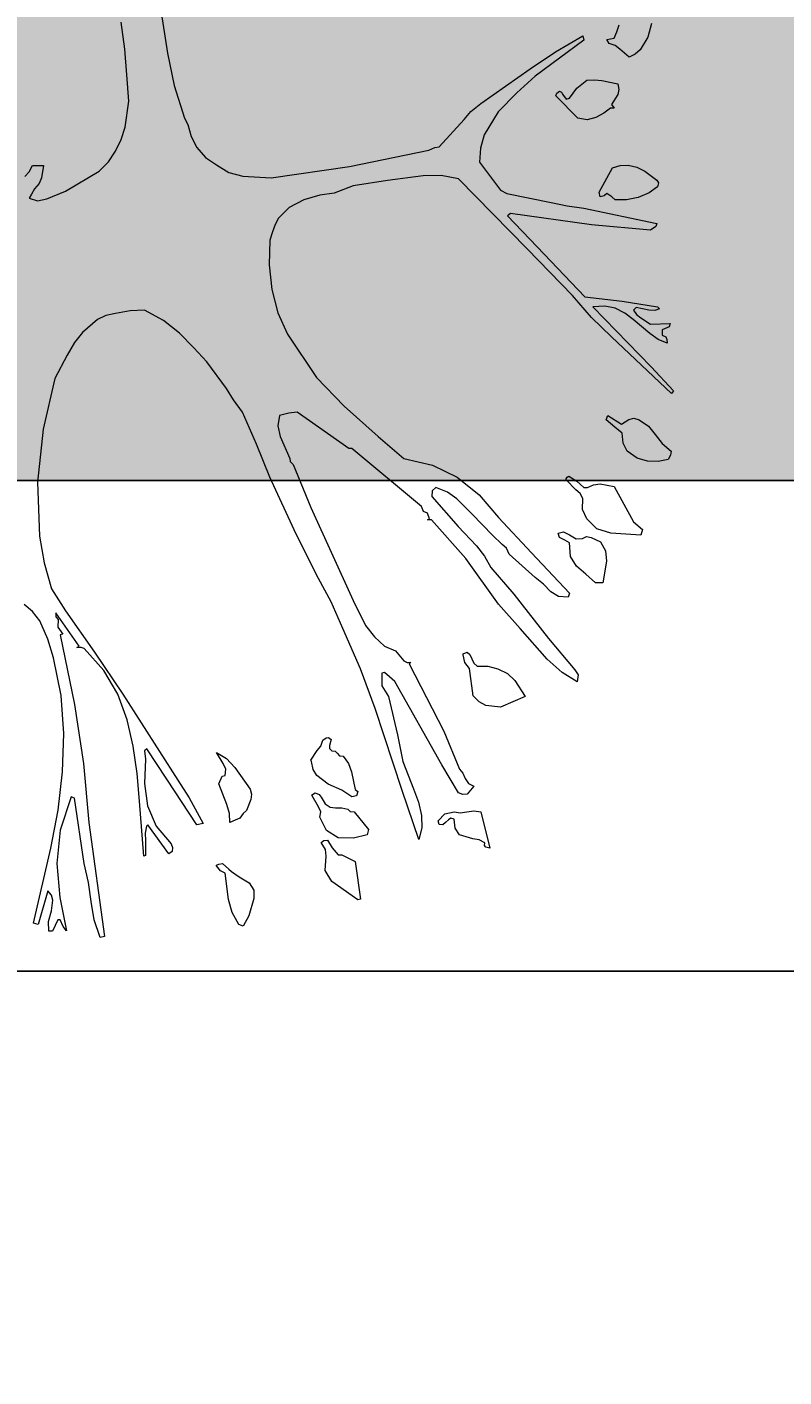
# Model space of a CAD drawing. Units: inches. Extents: x 84 to 1044, y -280 to 906.
# Tile 28 of 105: x 775 to 789, y -129 to -105. Entities that reach past the tile are written whole.
import ezdxf

# ---------------------------------------------------------------- set-up
doc = ezdxf.new("R2010")
doc.units = ezdxf.units.IN
for name, color, linetype, lineweight in [('A-ANNO-DIMS', 2, 'Continuous', 18), ('C-PROP', 7, 'Continuous', 25), ('L-PLNT', 114, 'Continuous', 15)]:
    doc.layers.add(name, color=color, linetype=linetype, lineweight=lineweight)
doc.layers.add('L-PLNT-PATT', color=9, linetype='Continuous', lineweight=9, true_color=0xafd9aa)
doc.styles.get("Standard").update_dxf_attribs({"font": 'arial.ttf'})
doc.dimstyles.get("Standard").update_dxf_attribs({"dimtxt": 0.18, "dimasz": 0.18, "dimexe": 0.18, "dimexo": 0.0625, "dimgap": 0.09, "dimtad": 0, "dimtih": 1, "dimtoh": 1, "dimdec": 4, "dimzin": 0, "dimdsep": 46, "dimtxsty": 'Standard', "dimcen": 0.09, "dimadec": 0, "dimazin": 0, "dimtfac": 1, "dimtdec": 4, "dimtofl": 0, "dimtmove": 0, "dimatfit": 3, "dimfxl": 1, "dimtolj": 1, "dimtzin": 0, "dimarcsym": 0})

# ---------------------------------------------------------------- blocks, each defined once
blk = doc.blocks.new('A$C37E508DF')
for p, q in [((0.7911, 1.1436), (0.8027, 1.0677)), ((0.7512, 1.0728), (0.7469, 1.1054)), ((1.3421, 1.0861), (1.3455, 1.0934)), ((1.3455, 1.0934), (1.3485, 1.102)), ((1.3875, 1.1037), (1.3828, 1.087)), ((1.3057, 1.0835), (1.2469, 1.0402)), ((1.2713, 1.0694), (1.3044, 1.0887)), ((1.3044, 1.0887), (1.3057, 1.0835)), ((1.3335, 1.0844), (1.3421, 1.0861)), ((1.3361, 1.0793), (1.3335, 1.0844)), ((1.3434, 1.0771), (1.3361, 1.0793)), ((1.349, 1.0728), (1.3434, 1.0771)), ((1.3828, 1.087), (1.3738, 1.072)), ((0.7538, 1.0415), (0.7512, 1.0728)), ((0.8027, 1.0677), (0.8108, 1.0287)), ((1.2409, 1.0488), (1.2713, 1.0694)), ((1.3605, 1.063), (1.349, 1.0728)), ((1.3678, 1.0664), (1.3605, 1.063)), ((1.3738, 1.072), (1.3678, 1.0664)), ((1.1813, 1.0072), (1.2409, 1.0488)), ((0.7559, 1.0098), (0.7538, 1.0415)), ((0.8108, 1.0287), (0.8233, 0.9892)), ((1.2469, 1.0402), (1.2246, 1.0201)), ((1.2971, 1.0257), (1.3091, 1.0351)), ((1.3091, 1.0351), (1.3185, 1.0355)), ((1.3185, 1.0355), (1.3275, 1.0347)), ((1.3275, 1.0347), (1.3468, 1.0308)), ((1.3468, 1.0308), (1.3481, 1.0239)), ((1.2246, 1.0201), (1.2023, 0.9969)), ((1.2718, 1.0162), (1.2731, 1.0197)), ((1.2984, 0.9892), (1.2718, 1.0162)), ((1.2731, 1.0197), (1.2761, 1.0218)), ((1.2761, 1.0218), (1.2786, 1.0209)), ((1.2786, 1.0209), (1.2799, 1.0184)), ((1.2799, 1.0184), (1.2842, 1.0124)), ((1.2842, 1.0124), (1.2885, 1.0136)), ((1.2885, 1.0136), (1.2971, 1.0257)), ((1.3468, 1.018), (1.3391, 1.0059)), ((1.3481, 1.0239), (1.3468, 1.018)), ((0.7516, 0.9785), (0.7559, 1.0098)), ((1.1612, 0.9879), (1.1693, 0.9974)), ((1.1693, 0.9974), (1.1813, 1.0072)), ((1.2023, 0.9969), (1.1852, 0.9691)), ((1.3297, 0.9952), (1.3202, 0.9901)), ((1.3378, 1.0016), (1.3297, 0.9952)), ((1.3421, 1.0016), (1.3378, 1.0016)), ((1.3391, 1.0059), (1.3421, 1.0016)), ((0.7469, 0.9635), (0.7516, 0.9785)), ((0.8233, 0.9892), (0.8275, 0.9815)), ((0.8275, 0.9815), (0.8314, 0.9673)), ((1.1311, 0.9549), (1.1612, 0.9879)), ((1.3095, 0.9875), (1.2984, 0.9892)), ((1.3202, 0.9901), (1.3095, 0.9875)), ((0.7401, 0.9493), (0.7469, 0.9635)), ((0.8314, 0.9673), (0.8383, 0.954)), ((1.1852, 0.9691), (1.1809, 0.9532)), ((0.7315, 0.9365), (0.7401, 0.9493)), ((0.8383, 0.954), (0.8486, 0.942)), ((1.0227, 0.9309), (1.1183, 0.9506)), ((1.1183, 0.9506), (1.1256, 0.954)), ((1.1256, 0.954), (1.1311, 0.9549)), ((1.1809, 0.9532), (1.1796, 0.936)), ((0.6359, 0.9245), (0.6397, 0.9322)), ((0.6397, 0.9322), (0.653, 0.9322)), ((0.653, 0.9322), (0.6505, 0.9172)), ((0.7203, 0.9253), (0.7315, 0.9365)), ((0.8486, 0.942), (0.8619, 0.933)), ((0.8619, 0.933), (0.8769, 0.9236)), ((0.9279, 0.9172), (1.0227, 0.9309)), ((1.1796, 0.936), (1.2049, 0.9022)), ((1.3241, 0.9), (1.3404, 0.9292)), ((1.3404, 0.9292), (1.3494, 0.9322)), ((1.3494, 0.9322), (1.3592, 0.9326)), ((1.3592, 0.9326), (1.3695, 0.93)), ((1.3695, 0.93), (1.3794, 0.9253)), ((0.6303, 0.9189), (0.6359, 0.9245)), ((0.6505, 0.9172), (0.6479, 0.9103)), ((0.6796, 0.9013), (0.7203, 0.9253)), ((0.8769, 0.9236), (0.8936, 0.9193)), ((0.8936, 0.9193), (0.9279, 0.9172)), ((1.0685, 0.9142), (1.0269, 0.9077)), ((1.1114, 0.9198), (1.0685, 0.9142)), ((1.1333, 0.9202), (1.1114, 0.9198)), ((1.1543, 0.9159), (1.1333, 0.9202)), ((1.2371, 0.8314), (1.1543, 0.9159)), ((1.3794, 0.9253), (1.394, 0.9146)), ((1.394, 0.9146), (1.3957, 0.9112)), ((0.6384, 0.8974), (0.6359, 0.8927)), ((0.6423, 0.9039), (0.6384, 0.8974)), ((0.6479, 0.9103), (0.6423, 0.9039)), ((0.6569, 0.8919), (0.6796, 0.9013)), ((1.0042, 0.8987), (0.9866, 0.8962)), ((1.0269, 0.9077), (1.0042, 0.8987)), ((1.2049, 0.9022), (1.2126, 0.8983)), ((1.2126, 0.8983), (1.2662, 0.8876)), ((1.3254, 0.8944), (1.3241, 0.9)), ((1.3335, 0.8983), (1.3301, 0.8957)), ((1.3395, 0.8944), (1.3335, 0.8983)), ((1.3846, 0.8992), (1.3713, 0.8936)), ((1.3948, 0.9065), (1.3846, 0.8992)), ((1.3957, 0.9112), (1.3948, 0.9065)), ((0.6359, 0.8927), (0.6457, 0.8897)), ((0.6457, 0.8897), (0.6569, 0.8919)), ((0.9498, 0.8816), (0.9369, 0.8687)), ((0.9673, 0.8906), (0.9498, 0.8816)), ((0.9866, 0.8962), (0.9673, 0.8906)), ((1.2662, 0.8876), (1.2855, 0.8833)), ((1.2855, 0.8833), (1.3057, 0.8807)), ((1.3057, 0.8807), (1.394, 0.8623)), ((1.3301, 0.8957), (1.3254, 0.8944)), ((1.3434, 0.8906), (1.3395, 0.8944)), ((1.3571, 0.8906), (1.3434, 0.8906)), ((1.3713, 0.8936), (1.3571, 0.8906)), ((0.9369, 0.8687), (0.933, 0.861)), ((1.2169, 0.8743), (1.2135, 0.8713)), ((1.2135, 0.8713), (1.2491, 0.834)), ((1.3151, 0.8606), (1.2169, 0.8743)), ((0.9296, 0.852), (0.9262, 0.8421)), ((0.933, 0.861), (0.9296, 0.852)), ((1.3863, 0.8541), (1.3151, 0.8606)), ((1.3927, 0.8584), (1.3863, 0.8541)), ((1.394, 0.8623), (1.3927, 0.8584)), ((0.9262, 0.8421), (0.9257, 0.8121)), ((1.2919, 0.7752), (1.2371, 0.8314)), ((1.2491, 0.834), (1.3069, 0.7735)), ((0.9257, 0.8121), (0.9287, 0.7825)), ((0.9287, 0.7825), (0.936, 0.7542)), ((1.3151, 0.7487), (1.2919, 0.7752)), ((1.3069, 0.7735), (1.352, 0.7684)), ((1.352, 0.7684), (1.3948, 0.7615)), ((0.7285, 0.7512), (0.7182, 0.7461)), ((0.7401, 0.7534), (0.7285, 0.7512)), ((0.7577, 0.7568), (0.7401, 0.7534)), ((0.7752, 0.7577), (0.7577, 0.7568)), ((0.798, 0.7452), (0.7752, 0.7577)), ((0.936, 0.7542), (0.9476, 0.7285)), ((1.3309, 0.7624), (1.3164, 0.7615)), ((1.3164, 0.7615), (1.3871, 0.6891)), ((1.3434, 0.7598), (1.3309, 0.7624)), ((1.355, 0.7538), (1.3434, 0.7598)), ((1.3653, 0.7461), (1.355, 0.7538)), ((1.3687, 0.7607), (1.3657, 0.7577)), ((1.3657, 0.7577), (1.3691, 0.7521)), ((1.3841, 0.7577), (1.3687, 0.7607)), ((1.3691, 0.7521), (1.3743, 0.7482)), ((1.3914, 0.7572), (1.3841, 0.7577)), ((1.397, 0.759), (1.3914, 0.7572)), ((1.3948, 0.7615), (1.397, 0.759)), ((0.7182, 0.7461), (0.7002, 0.7307)), ((0.8173, 0.7298), (0.798, 0.7452)), ((1.3391, 0.7255), (1.3151, 0.7487)), ((1.3854, 0.7294), (1.3653, 0.7461)), ((1.3743, 0.7482), (1.3863, 0.7405)), ((1.3863, 0.7405), (1.4099, 0.7414)), ((1.4086, 0.7375), (1.4004, 0.7337)), ((1.4004, 0.7337), (1.4004, 0.7272)), ((1.4099, 0.7414), (1.4086, 0.7375)), ((0.6903, 0.7186), (0.6818, 0.7032)), ((0.7002, 0.7307), (0.6903, 0.7186)), ((0.8344, 0.7122), (0.8173, 0.7298)), ((0.9476, 0.7285), (0.9828, 0.6762)), ((1.4116, 0.6569), (1.3391, 0.7255)), ((1.3953, 0.7221), (1.3854, 0.7294)), ((1.4064, 0.7178), (1.3953, 0.7221)), ((1.4004, 0.7272), (1.4047, 0.7255)), ((1.4047, 0.7255), (1.406, 0.7221)), ((1.406, 0.7221), (1.4064, 0.7178)), ((0.6818, 0.7032), (0.6667, 0.6749)), ((0.8503, 0.6951), (0.8344, 0.7122)), ((0.8739, 0.6629), (0.8503, 0.6951)), ((1.3871, 0.6891), (1.4141, 0.6599)), ((0.6667, 0.6749), (0.6526, 0.614)), ((0.9828, 0.6762), (1.0162, 0.6415)), ((0.8824, 0.6492), (0.8739, 0.6629)), ((1.4141, 0.6599), (1.4116, 0.6569)), ((0.8932, 0.6342), (0.8824, 0.6492)), ((1.0162, 0.6415), (1.0574, 0.605)), ((0.9103, 0.5956), (0.8932, 0.6342)), ((0.9382, 0.6303), (0.936, 0.6179)), ((0.9493, 0.6333), (0.9382, 0.6303)), ((0.9596, 0.6342), (0.9493, 0.6333)), ((1.0218, 0.5904), (0.9596, 0.6342)), ((1.3327, 0.6252), (1.3348, 0.6303)), ((1.343, 0.6162), (1.3327, 0.6252)), ((1.3348, 0.6303), (1.3511, 0.62)), ((1.3511, 0.62), (1.3601, 0.6256)), ((1.3601, 0.6256), (1.3661, 0.6269)), ((1.3661, 0.6269), (1.3725, 0.6252)), ((1.3725, 0.6252), (1.3837, 0.6175)), ((0.6526, 0.614), (0.6457, 0.5497)), ((0.936, 0.6179), (0.939, 0.605)), ((0.939, 0.605), (0.9506, 0.5784)), ((1.0574, 0.605), (1.0883, 0.5784)), ((1.352, 0.6089), (1.343, 0.6162)), ((1.3533, 0.5969), (1.352, 0.6089)), ((1.3837, 0.6175), (1.3918, 0.6072)), ((1.3918, 0.6072), (1.4004, 0.5964)), ((0.9262, 0.5557), (0.9103, 0.5956)), ((1.0256, 0.5904), (1.0218, 0.5904)), ((1.1097, 0.5205), (1.0256, 0.5904)), ((1.358, 0.5874), (1.3533, 0.5969)), ((1.37, 0.5789), (1.358, 0.5874)), ((1.4004, 0.5964), (1.4111, 0.5874)), ((1.4111, 0.5874), (1.4103, 0.5823)), ((0.9506, 0.5784), (0.951, 0.5746)), ((0.951, 0.5746), (0.9545, 0.5711)), ((0.9545, 0.5711), (0.9759, 0.5193)), ((1.0883, 0.5784), (1.123, 0.5703)), ((1.3824, 0.575), (1.37, 0.5789)), ((1.3953, 0.5746), (1.3824, 0.575)), ((1.4077, 0.5771), (1.3953, 0.5746)), ((1.4103, 0.5823), (1.4077, 0.5771)), ((0.9583, 0.4871), (0.9262, 0.5557)), ((1.123, 0.5703), (1.1526, 0.5557)), ((1.1526, 0.5557), (1.1792, 0.5347)), ((1.2842, 0.554), (1.2855, 0.5557)), ((1.2855, 0.5557), (1.2876, 0.557)), ((1.2876, 0.557), (1.2971, 0.551)), ((0.6457, 0.5497), (0.6483, 0.4845)), ((1.1226, 0.5394), (1.1221, 0.5325)), ((1.1268, 0.5433), (1.1226, 0.5394)), ((1.141, 0.5377), (1.1268, 0.5433)), ((1.2842, 0.5527), (1.2842, 0.554)), ((1.2958, 0.5407), (1.2842, 0.5527)), ((1.3014, 0.536), (1.2958, 0.5407)), ((1.2971, 0.551), (1.3057, 0.5433)), ((1.3057, 0.5433), (1.3099, 0.5433)), ((1.3099, 0.5433), (1.3172, 0.5467)), ((1.3172, 0.5467), (1.3254, 0.548)), ((1.3254, 0.548), (1.3421, 0.5446)), ((1.3421, 0.5446), (1.3657, 0.5021)), ((1.1221, 0.5325), (1.1539, 0.4961)), ((1.1521, 0.5296), (1.141, 0.5377)), ((1.1706, 0.5111), (1.1521, 0.5296)), ((1.1792, 0.5347), (1.2027, 0.5072)), ((1.3044, 0.53), (1.3014, 0.536)), ((1.3039, 0.5167), (1.3044, 0.53)), ((0.9759, 0.5193), (1.0269, 0.4069)), ((1.1118, 0.5145), (1.1097, 0.5205)), ((1.117, 0.5124), (1.1118, 0.5145)), ((1.1191, 0.5055), (1.117, 0.5124)), ((1.117, 0.5042), (1.1191, 0.5055)), ((1.1955, 0.4858), (1.1706, 0.5111)), ((1.2027, 0.5072), (1.2426, 0.4644)), ((1.3091, 0.5055), (1.3039, 0.5167)), ((1.3215, 0.4935), (1.3091, 0.5055)), ((1.1217, 0.5042), (1.117, 0.5042)), ((1.1633, 0.4575), (1.1217, 0.5042)), ((1.1539, 0.4961), (1.1762, 0.4729)), ((1.2748, 0.4884), (1.2812, 0.4897)), ((1.2812, 0.4897), (1.2885, 0.4862)), ((1.3382, 0.4884), (1.3215, 0.4935)), ((1.3657, 0.5021), (1.3764, 0.4927)), ((1.3764, 0.4927), (1.3743, 0.4858)), ((0.6483, 0.4845), (0.6539, 0.4524)), ((0.9853, 0.4335), (0.9583, 0.4871)), ((1.1762, 0.4729), (1.1856, 0.4605)), ((1.207, 0.4747), (1.1955, 0.4858)), ((1.2122, 0.47), (1.207, 0.4747)), ((1.2761, 0.4832), (1.2748, 0.4884)), ((1.2825, 0.4798), (1.2761, 0.4832)), ((1.2885, 0.4764), (1.2825, 0.4798)), ((1.2885, 0.4862), (1.2962, 0.4815)), ((1.2894, 0.4601), (1.2885, 0.4764)), ((1.2962, 0.4815), (1.3039, 0.482)), ((1.3039, 0.482), (1.3087, 0.4841)), ((1.3087, 0.4841), (1.3147, 0.4832)), ((1.3147, 0.4832), (1.3258, 0.4777)), ((1.3258, 0.4777), (1.3318, 0.4669)), ((1.3743, 0.4858), (1.3382, 0.4884)), ((1.2027, 0.4026), (1.1633, 0.4575)), ((1.1856, 0.4605), (1.1933, 0.4468)), ((1.2156, 0.4627), (1.2122, 0.47)), ((1.2469, 0.4348), (1.2156, 0.4627)), ((1.2426, 0.4644), (1.2885, 0.4159)), ((1.2967, 0.4485), (1.2894, 0.4601)), ((1.3318, 0.4669), (1.3331, 0.4545)), ((0.6539, 0.4524), (0.6625, 0.4211)), ((1.1933, 0.4468), (1.2212, 0.4146)), ((1.3082, 0.4386), (1.2967, 0.4485)), ((1.3331, 0.4545), (1.3284, 0.4284)), ((1.0003, 0.4052), (0.9853, 0.4335)), ((1.2568, 0.4266), (1.2469, 0.4348)), ((1.2658, 0.4176), (1.2568, 0.4266)), ((1.3198, 0.4284), (1.3082, 0.4386)), ((1.3284, 0.4284), (1.3198, 0.4284)), ((0.6625, 0.4211), (0.6796, 0.3945)), ((1.2212, 0.4146), (1.2628, 0.361)), ((1.2752, 0.4116), (1.2658, 0.4176)), ((1.2868, 0.4108), (1.2752, 0.4116)), ((1.2885, 0.4159), (1.2868, 0.4108)), ((0.6397, 0.3936), (0.6295, 0.4022)), ((0.6487, 0.3825), (0.6397, 0.3936)), ((0.6959, 0.352), (0.668, 0.3919)), ((0.668, 0.3919), (0.668, 0.3872)), ((0.6796, 0.3945), (0.7148, 0.3447)), ((1.0145, 0.373), (1.0003, 0.4052)), ((1.0269, 0.4069), (1.0419, 0.3769)), ((1.2289, 0.373), (1.2027, 0.4026)), ((0.6582, 0.3602), (0.6487, 0.3825)), ((0.668, 0.3872), (0.6706, 0.3842)), ((0.6706, 0.3842), (0.6702, 0.3748)), ((1.0419, 0.3769), (1.0527, 0.3632)), ((0.665, 0.3379), (0.6582, 0.3602)), ((0.6702, 0.3748), (0.6762, 0.3662)), ((0.6762, 0.3662), (0.6732, 0.3653)), ((0.6732, 0.3653), (0.6903, 0.2813)), ((1.0359, 0.3246), (1.0145, 0.373)), ((1.0527, 0.3632), (1.0647, 0.352)), ((1.2615, 0.3362), (1.2289, 0.373)), ((1.2628, 0.361), (1.2949, 0.3233)), ((0.6933, 0.3503), (0.6959, 0.352)), ((0.6985, 0.3503), (0.6933, 0.3503)), ((0.7023, 0.349), (0.6985, 0.3503)), ((0.7259, 0.3224), (0.7023, 0.349)), ((0.7148, 0.3447), (0.7487, 0.2937)), ((1.0647, 0.352), (1.078, 0.346)), ((1.078, 0.346), (1.0883, 0.334)), ((1.1599, 0.3426), (1.1646, 0.3447)), ((1.1599, 0.3413), (1.1599, 0.3426)), ((1.1646, 0.3447), (1.168, 0.3417)), ((0.6745, 0.2924), (0.665, 0.3379)), ((1.0883, 0.334), (1.0921, 0.3319)), ((1.0921, 0.3319), (1.0968, 0.3319)), ((1.0968, 0.3319), (1.0947, 0.3306)), ((1.0947, 0.3306), (1.1367, 0.2491)), ((1.162, 0.3319), (1.1599, 0.3413)), ((1.1676, 0.325), (1.162, 0.3319)), ((1.168, 0.3417), (1.1702, 0.3366)), ((1.1702, 0.3366), (1.1727, 0.3314)), ((1.1727, 0.3314), (1.177, 0.3276)), ((1.177, 0.3276), (1.1895, 0.3276)), ((1.1895, 0.3276), (1.2019, 0.3246)), ((1.2795, 0.3199), (1.2615, 0.3362)), ((0.7427, 0.2937), (0.7259, 0.3224)), ((1.0535, 0.2766), (1.0359, 0.3246)), ((1.0647, 0.3199), (1.0617, 0.3194)), ((1.0617, 0.3194), (1.0617, 0.304)), ((1.0711, 0.3147), (1.0647, 0.3199)), ((1.0775, 0.3092), (1.0711, 0.3147)), ((1.1719, 0.292), (1.1676, 0.325)), ((1.2019, 0.3246), (1.2135, 0.3186)), ((1.2135, 0.3186), (1.2225, 0.3104)), ((1.2225, 0.3104), (1.2349, 0.2911)), ((1.2975, 0.3087), (1.2795, 0.3199)), ((1.2949, 0.3233), (1.2988, 0.3173)), ((1.2988, 0.3173), (1.2975, 0.3087)), ((0.7542, 0.2628), (0.7427, 0.2937)), ((0.7487, 0.2937), (0.8151, 0.1899)), ((1.0617, 0.304), (1.0698, 0.2911)), ((1.1341, 0.2084), (1.0775, 0.3092)), ((0.6775, 0.2465), (0.6745, 0.2924)), ((0.6903, 0.2813), (0.7015, 0.2101)), ((1.0698, 0.2911), (1.0805, 0.2448)), ((1.1792, 0.2847), (1.1719, 0.292)), ((1.1873, 0.28), (1.1792, 0.2847)), ((1.2049, 0.2783), (1.1873, 0.28)), ((1.2349, 0.2911), (1.2049, 0.2783)), ((0.7615, 0.2311), (0.7542, 0.2628)), ((1.0861, 0.1775), (1.0535, 0.2766)), ((0.6758, 0.2002), (0.6775, 0.2465)), ((1.0805, 0.2448), (1.087, 0.2127)), ((1.1367, 0.2491), (1.1556, 0.2032)), ((0.7662, 0.1981), (0.7615, 0.2311)), ((0.9836, 0.226), (0.9879, 0.2311)), ((0.9879, 0.2311), (0.9905, 0.2384)), ((0.9905, 0.2384), (0.9943, 0.241)), ((0.9943, 0.241), (0.9973, 0.2414)), ((0.9973, 0.2414), (1.0003, 0.2393)), ((1.0003, 0.2393), (0.9986, 0.232)), ((0.9986, 0.232), (0.9986, 0.2281)), ((0.7778, 0.2277), (0.7752, 0.2255)), ((0.7752, 0.2255), (0.7761, 0.2152)), ((0.7761, 0.2152), (0.7752, 0.1861)), ((0.8018, 0.1912), (0.7778, 0.2277)), ((0.8619, 0.2234), (0.8739, 0.2161)), ((0.87, 0.2101), (0.8619, 0.2234)), ((0.8739, 0.2161), (0.8841, 0.2054)), ((0.9759, 0.214), (0.9836, 0.226)), ((0.9768, 0.2127), (0.9759, 0.214)), ((0.9789, 0.2028), (0.9768, 0.2127)), ((0.9986, 0.2281), (1.0012, 0.2255)), ((1.0012, 0.2255), (1.0051, 0.2251)), ((1.0051, 0.2251), (1.0076, 0.2225)), ((1.0076, 0.2225), (1.0106, 0.2195)), ((1.0106, 0.2195), (1.0149, 0.2191)), ((1.0149, 0.2191), (1.0214, 0.2101)), ((1.087, 0.2127), (1.0998, 0.1797)), ((0.6706, 0.1539), (0.6758, 0.2002)), ((0.7015, 0.2101), (0.7079, 0.1389)), ((0.7688, 0.1646), (0.7662, 0.1981)), ((0.8734, 0.2032), (0.87, 0.2101)), ((0.8726, 0.1955), (0.8734, 0.2032)), ((0.8841, 0.2054), (0.9026, 0.1792)), ((0.9832, 0.1955), (0.9789, 0.2028)), ((1.0214, 0.2101), (1.0252, 0.2002)), ((1.0252, 0.2002), (1.0295, 0.1788)), ((1.1543, 0.1749), (1.1341, 0.2084)), ((1.1556, 0.2032), (1.1594, 0.1985)), ((1.1594, 0.1985), (1.1624, 0.1921)), ((0.7752, 0.1861), (0.7787, 0.1591)), ((0.8383, 0.1359), (0.8018, 0.1912)), ((0.8151, 0.1899), (0.8288, 0.1685)), ((0.8649, 0.1857), (0.8687, 0.1947)), ((0.8743, 0.1608), (0.8649, 0.1857)), ((0.8687, 0.1947), (0.8726, 0.1955)), ((0.9969, 0.1852), (0.9832, 0.1955)), ((1.0132, 0.1779), (0.9969, 0.1852)), ((1.0998, 0.1797), (1.1058, 0.1634)), ((1.1624, 0.1921), (1.1663, 0.1861)), ((1.1727, 0.1827), (1.1646, 0.1732)), ((1.1663, 0.1861), (1.1727, 0.1827)), ((0.6865, 0.1698), (0.6732, 0.1295)), ((0.6903, 0.1681), (0.6865, 0.1698)), ((0.7023, 0.0892), (0.6903, 0.1681)), ((0.774, 0.0982), (0.7688, 0.1646)), ((0.8288, 0.1685), (0.846, 0.1376)), ((0.9035, 0.1668), (0.8983, 0.1535)), ((0.9026, 0.1792), (0.9043, 0.1732)), ((0.9043, 0.1732), (0.9035, 0.1668)), ((0.9768, 0.1719), (0.9811, 0.1749)), ((0.9776, 0.1711), (0.9768, 0.1719)), ((0.9853, 0.1578), (0.9776, 0.1711)), ((0.9811, 0.1749), (0.9858, 0.1728)), ((0.9858, 0.1728), (0.9884, 0.1694)), ((0.9884, 0.1694), (0.9931, 0.1616)), ((1.0256, 0.1698), (1.0132, 0.1779)), ((1.0312, 0.1711), (1.0256, 0.1698)), ((1.0295, 0.1788), (1.0325, 0.1762)), ((1.0325, 0.1762), (1.0312, 0.1711)), ((1.1063, 0.1183), (1.0861, 0.1775)), ((1.1058, 0.1634), (1.1097, 0.1475)), ((1.1594, 0.1728), (1.1543, 0.1749)), ((1.1646, 0.1732), (1.1594, 0.1728)), ((0.662, 0.108), (0.6706, 0.1539)), ((0.7787, 0.1591), (0.789, 0.1346)), ((0.8777, 0.1496), (0.8743, 0.1608)), ((0.8781, 0.1389), (0.8777, 0.1496)), ((0.894, 0.1496), (0.8902, 0.1441)), ((0.8983, 0.1535), (0.894, 0.1496)), ((0.9879, 0.1518), (0.9853, 0.1578)), ((0.9866, 0.1453), (0.9879, 0.1518)), ((0.9931, 0.1616), (0.9991, 0.1574)), ((0.9991, 0.1574), (1.0059, 0.1565)), ((1.0059, 0.1565), (1.0132, 0.1565)), ((1.0132, 0.1565), (1.0205, 0.1548)), ((1.0205, 0.1548), (1.0235, 0.1522)), ((1.0235, 0.1522), (1.0282, 0.1518)), ((1.0282, 0.1518), (1.0454, 0.1303)), ((1.1097, 0.1475), (1.1101, 0.1325)), ((1.1298, 0.1411), (1.1376, 0.1492)), ((1.1376, 0.1492), (1.1491, 0.1518)), ((1.1491, 0.1518), (1.1564, 0.1505)), ((1.1564, 0.1505), (1.1642, 0.1518)), ((1.1642, 0.1518), (1.1727, 0.1531)), ((1.1727, 0.1531), (1.1813, 0.1518)), ((1.1813, 0.1518), (1.192, 0.108)), ((0.7079, 0.1389), (0.7268, 0.0013)), ((0.7774, 0.1346), (0.7757, 0.1261)), ((0.7791, 0.1359), (0.7774, 0.1346)), ((0.8044, 0.1012), (0.7791, 0.1359)), ((0.789, 0.1346), (0.8074, 0.1132)), ((0.846, 0.1376), (0.8383, 0.1359)), ((0.8846, 0.1419), (0.8781, 0.1389)), ((0.8902, 0.1441), (0.8846, 0.1419)), ((0.9948, 0.1291), (0.9866, 0.1453)), ((1.1101, 0.1325), (1.1063, 0.1183)), ((1.1311, 0.1364), (1.1298, 0.1411)), ((1.1354, 0.1359), (1.1311, 0.1364)), ((1.1384, 0.1389), (1.1354, 0.1359)), ((1.1423, 0.1423), (1.1384, 0.1389)), ((1.1449, 0.1441), (1.1423, 0.1423)), ((1.1491, 0.1428), (1.1449, 0.1441)), ((1.1504, 0.132), (1.1491, 0.1428)), ((1.1556, 0.1239), (1.1504, 0.132)), ((0.6732, 0.1295), (0.6693, 0.0892)), ((0.7757, 0.1261), (0.7761, 0.117)), ((0.7761, 0.117), (0.7761, 0.099)), ((0.9884, 0.1149), (0.9918, 0.117)), ((0.9935, 0.1063), (0.9884, 0.1149)), ((0.9918, 0.117), (0.9961, 0.1175)), ((1.0089, 0.1205), (0.9948, 0.1291)), ((0.9961, 0.1175), (1.0016, 0.1085)), ((1.0274, 0.12), (1.0089, 0.1205)), ((1.0441, 0.1239), (1.0274, 0.12)), ((1.0454, 0.1303), (1.0441, 0.1239)), ((1.1714, 0.1192), (1.1556, 0.1239)), ((1.1792, 0.1179), (1.1714, 0.1192)), ((1.186, 0.1145), (1.1792, 0.1179)), ((1.1856, 0.111), (1.186, 0.1145)), ((0.641, 0.0172), (0.662, 0.108)), ((0.7761, 0.099), (0.774, 0.0982)), ((0.8083, 0.1037), (0.8044, 0.1012)), ((0.8074, 0.1132), (0.8087, 0.1089)), ((0.8087, 0.1089), (0.8083, 0.1037)), ((0.9931, 0.081), (0.9943, 0.0982)), ((0.9943, 0.0982), (0.9935, 0.1063)), ((1.0016, 0.1085), (1.0089, 0.0999)), ((1.0089, 0.0999), (1.0132, 0.0999)), ((1.0132, 0.0999), (1.0295, 0.0917)), ((1.1873, 0.1093), (1.1856, 0.111)), ((1.192, 0.108), (1.1873, 0.1093)), ((0.6693, 0.0892), (0.6728, 0.0484)), ((0.7075, 0.0665), (0.7023, 0.0892)), ((0.8619, 0.0875), (0.8649, 0.0887)), ((0.8619, 0.0866), (0.8619, 0.0875)), ((0.8666, 0.0806), (0.8619, 0.0866)), ((0.8649, 0.0887), (0.8691, 0.0892)), ((0.8691, 0.0892), (0.8769, 0.0827)), ((0.8769, 0.0827), (0.8799, 0.0797)), ((1.0295, 0.0917), (1.0359, 0.0463)), ((0.7105, 0.0437), (0.7075, 0.0665)), ((0.8726, 0.0776), (0.8666, 0.0806)), ((0.8764, 0.0459), (0.8726, 0.0776)), ((0.8799, 0.0797), (0.8893, 0.0733)), ((0.8893, 0.0733), (0.9013, 0.066)), ((0.9013, 0.066), (0.9069, 0.057)), ((1.0012, 0.0677), (0.9931, 0.081)), ((1.0325, 0.0454), (1.0012, 0.0677)), ((0.6582, 0.0562), (0.6466, 0.0159)), ((0.6625, 0.051), (0.6582, 0.0562)), ((0.6642, 0.045), (0.6625, 0.051)), ((0.9069, 0.057), (0.9069, 0.0471)), ((0.6625, 0.0321), (0.6642, 0.045)), ((0.6728, 0.0484), (0.6809, 0.0082)), ((0.7144, 0.0214), (0.7105, 0.0437)), ((0.8807, 0.0304), (0.8764, 0.0459)), ((0.9069, 0.0471), (0.9009, 0.0261)), ((1.0359, 0.0463), (1.0325, 0.0454)), ((0.6466, 0.0159), (0.641, 0.0172)), ((0.659, 0.0193), (0.6625, 0.0321)), ((0.6595, 0.0077), (0.659, 0.0193)), ((0.6702, 0.0214), (0.6637, 0.0077)), ((0.6732, 0.0214), (0.6702, 0.0214)), ((0.6766, 0.0133), (0.6732, 0.0214)), ((0.7216, 0), (0.7144, 0.0214)), ((0.8889, 0.0159), (0.8807, 0.0304)), ((0.9009, 0.0261), (0.894, 0.0137)), ((0.6637, 0.0077), (0.6595, 0.0077)), ((0.6809, 0.0082), (0.6766, 0.0133)), ((0.7268, 0.0013), (0.7216, 0)), ((0.894, 0.0137), (0.8889, 0.0159))]:
    blk.add_line(p, q)
blk = doc.blocks.new('*D60')
at = {"layer": 'A-ANNO-DIMS', "color": 0, "lineweight": -2, "transparency": 16777216}
for p, q in [((134.179, -121.942), (134.179, -180.64)), ((992.074, -121.942), (992.074, -180.64)), ((134.359, -180.46), (562.733, -180.46)), ((991.894, -180.46), (563.521, -180.46))]:
    blk.add_line(p, q, dxfattribs=at)
at = {"layer": 'A-ANNO-DIMS', "color": 0, "transparency": 16777216}
for points in [[(134.359, -180.43), (134.359, -180.49), (134.179, -180.46)], [(991.894, -180.43), (991.894, -180.49), (992.074, -180.46)]]:
    blk.add_solid(points, dxfattribs=at)
at = {"layer": 'Defpoints', "color": 0, "transparency": 16777216}
for p in [(134.179, -121.88), (992.074, -121.88), (992.074, -180.46)]:
    blk.add_point(p, dxfattribs=at)
at = {"layer": 'A-ANNO-DIMS', "color": 0, "transparency": 16777216, "insert": (563.127, -180.46), "char_height": 0.18, "attachment_point": 5}
blk.add_mtext('\\A1;857.9', dxfattribs=at)

msp = doc.modelspace()

# ---------------------------------------------------------------- hatches: boundary and pattern name
at = {"layer": 'L-PLNT-PATT', "transparency": 33554597}
h = msp.add_hatch(color=256, dxfattribs=at)
h.dxf.hatch_style = 1
h.paths.add_polyline_path([(791.074, 31.12), (791.074, 91.12), (743.074, 91.12), (674.074, 91.12), (674.074, 31.12), (650.074, 31.12), (650.074, -112.88), (983.074, -112.88), (983.074, -64.88), (791.074, -64.88)])

# ---------------------------------------------------------------- linework, layer by layer
at = {"layer": 'C-PROP'}
for points in [[(143.179, -121.88), (134.179, -121.88), (134.179, 856.12), (992.074, 856.12), (992.074, -121.88), (624.574, -121.88)], [(143.179, -112.88), (143.179, 847.12), (983.074, 847.12), (983.074, -112.88), (624.574, -112.88)]]:
    msp.add_lwpolyline(points, dxfattribs=at)

# ---------------------------------------------------------------- block references
at = {"layer": 'L-PLNT', "xscale": 15.19586232982809, "yscale": 15.19586232982809, "zscale": 15.19586232982809}
msp.add_blockref('A$C37E508DF', (765.534, -121.265), dxfattribs=at)

# ---------------------------------------------------------------- dimensions: what is measured, and where the dimension line sits
at = {"layer": 'A-ANNO-DIMS'}
dim = msp.add_linear_dim(base=(992.074, -180.46), p1=(134.179, -121.88), p2=(992.074, -121.88), dimstyle='Standard', override={"dimdec": 1, "dimlfac": 1, "dimrnd": 0, "dimzin": 0, "dimdsep": 46, "dimlunit": 2}, dxfattribs=at)
dim.commit()
dim.dimension.update_dxf_attribs({"geometry": '*D60', "text_midpoint": (563.127, -180.46)})

doc.saveas('drawing.dxf')
